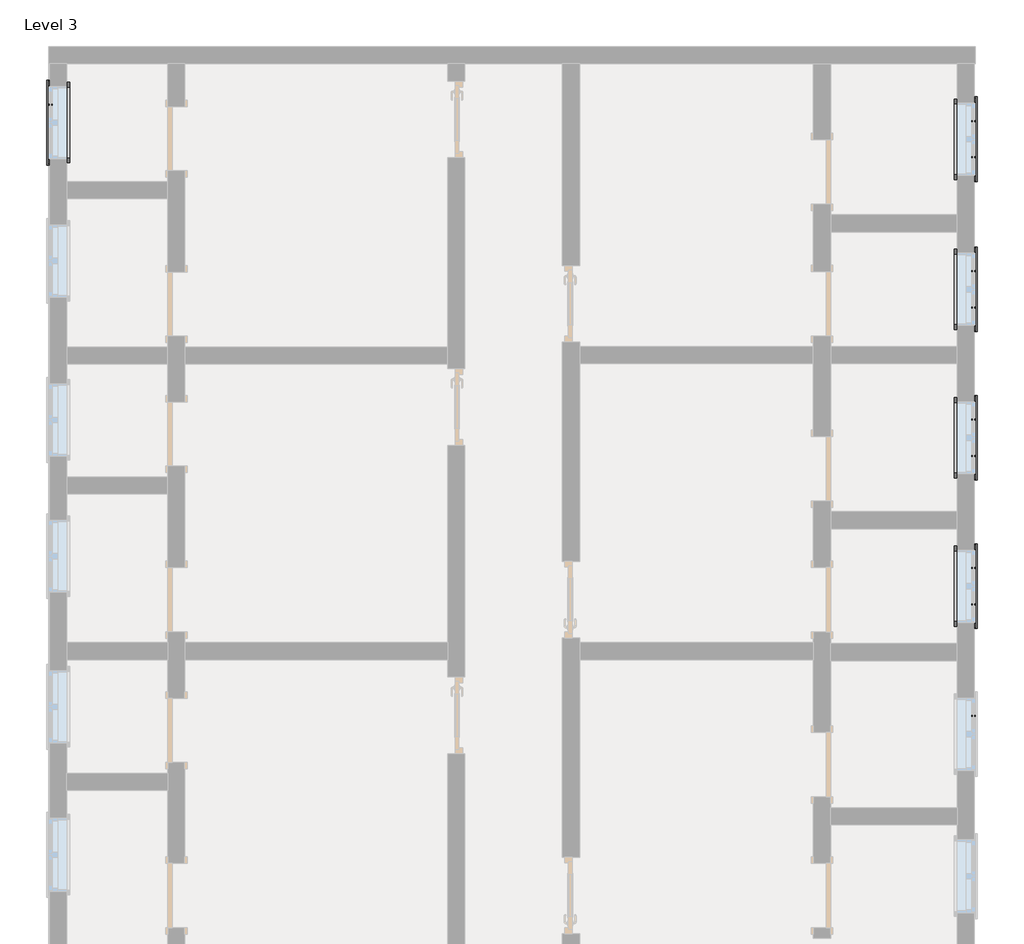
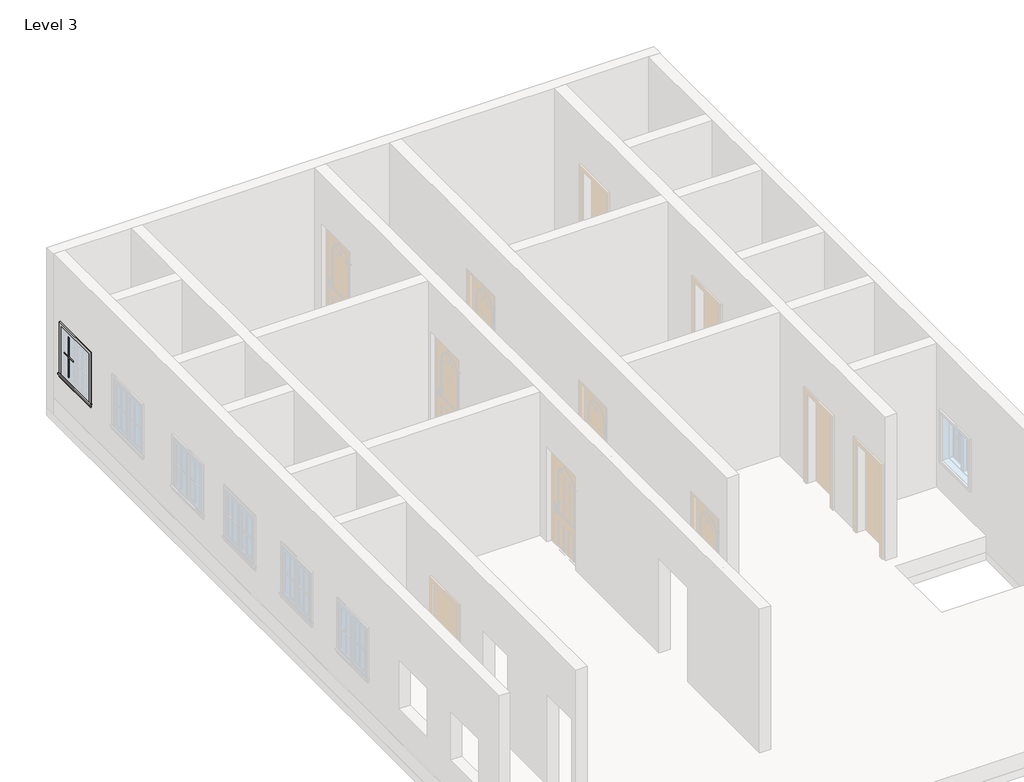
# One storey, part 4 of 4: 20 proxies.
"""IFC4 building model written with IfcOpenShell, lengths in millimetres."""

from ifc_helpers import new_model, si_unit, origin, place, context, project, spatial, transform, mapped, element, save
from components import muntin_pattern_2x2_muntin_pattern_2x2_b3fe6957, muntin_pattern_2x2_muntin_pattern_2x2_3e0ecaf2, trim_window_exterior_flat_with_sill_41619996, trim_window_interior_flat_picture_frame_51c85655

model = new_model("IFC4")

# Units and contexts
model_context = context("Model", 3, world=origin())
ifc_project = project(units=[si_unit("LENGTHUNIT", "METRE", prefix="MILLI")], contexts=[model_context])

# Site, building, storey
site = spatial("IfcSite", under=ifc_project)
building = spatial("IfcBuilding", under=site)
storey = spatial("IfcBuildingStorey", under=building, Name="Level 3", Elevation=6096.0)

# Proxies
placement = place(None, origin())
muntin_pattern_2x2_muntin_pattern_2x2_shape = muntin_pattern_2x2_muntin_pattern_2x2_b3fe6957(model_context)
element("IfcBuildingElementProxy", 1, Name="Muntin Pattern_2x2 : Muntin Pattern_2x2", ObjectType="Muntin Pattern_2x2 : Muntin Pattern_2x2", at=placement, inside=storey, context=model_context, shape_type="MappedRepresentation", body=[
    mapped(muntin_pattern_2x2_muntin_pattern_2x2_shape, transform((4489.4641134, 66.1024728, 7080.25), x_axis=(0.0, -1.0, 0.0), y_axis=(1.0, 0.0, 0.0), z_axis=(0.0, 0.0, 1.0))),
])
element("IfcBuildingElementProxy", 2, Name="Muntin Pattern_2x2 : Muntin Pattern_2x2", ObjectType="Muntin Pattern_2x2 : Muntin Pattern_2x2", at=placement, inside=storey, context=model_context, shape_type="MappedRepresentation", body=[
    mapped(muntin_pattern_2x2_muntin_pattern_2x2_shape, transform((4489.4641134, 1818.7024728, 7080.25), x_axis=(0.0, -1.0, 0.0), y_axis=(1.0, 0.0, 0.0), z_axis=(0.0, 0.0, 1.0))),
])
element("IfcBuildingElementProxy", 3, Name="Muntin Pattern_2x2 : Muntin Pattern_2x2", ObjectType="Muntin Pattern_2x2 : Muntin Pattern_2x2", at=placement, inside=storey, context=model_context, shape_type="MappedRepresentation", body=[
    mapped(muntin_pattern_2x2_muntin_pattern_2x2_shape, transform((4489.4641134, 3577.6524728, 7080.25), x_axis=(0.0, -1.0, 0.0), y_axis=(1.0, 0.0, 0.0), z_axis=(0.0, 0.0, 1.0))),
])
element("IfcBuildingElementProxy", 4, Name="Muntin Pattern_2x2 : Muntin Pattern_2x2", ObjectType="Muntin Pattern_2x2 : Muntin Pattern_2x2", at=placement, inside=storey, context=model_context, shape_type="MappedRepresentation", body=[
    mapped(muntin_pattern_2x2_muntin_pattern_2x2_shape, transform((4489.4641134, 5336.6024728, 7080.25), x_axis=(0.0, -1.0, 0.0), y_axis=(1.0, 0.0, 0.0), z_axis=(0.0, 0.0, 1.0))),
])
element("IfcBuildingElementProxy", 5, Name="Muntin Pattern_2x2 : Muntin Pattern_2x2", ObjectType="Muntin Pattern_2x2 : Muntin Pattern_2x2", at=placement, inside=storey, context=model_context, shape_type="MappedRepresentation", body=[
    mapped(muntin_pattern_2x2_muntin_pattern_2x2_shape, transform((4489.4641134, 7114.6024728, 7080.25), x_axis=(0.0, -1.0, 0.0), y_axis=(1.0, 0.0, 0.0), z_axis=(0.0, 0.0, 1.0))),
])
muntin_pattern_2x2_muntin_pattern_2x2_2_shape = muntin_pattern_2x2_muntin_pattern_2x2_3e0ecaf2(model_context)
element("IfcBuildingElementProxy", 6, Name="Muntin Pattern_2x2 : Muntin Pattern_2x2", ObjectType="Muntin Pattern_2x2 : Muntin Pattern_2x2", at=placement, inside=storey, context=model_context, shape_type="MappedRepresentation", body=[
    mapped(muntin_pattern_2x2_muntin_pattern_2x2_2_shape, transform((-6438.8858866, 7311.4524728, 7080.25), x_axis=(0.0, -1.0, 0.0), y_axis=(1.0, 0.0, 0.0), z_axis=(0.0, 0.0, 1.0))),
])
element("IfcBuildingElementProxy", 7, Name="Muntin Pattern_2x2 : Muntin Pattern_2x2", ObjectType="Muntin Pattern_2x2 : Muntin Pattern_2x2", at=placement, inside=storey, context=model_context, shape_type="MappedRepresentation", body=[
    mapped(muntin_pattern_2x2_muntin_pattern_2x2_2_shape, transform((4489.4641134, 1390.0774728, 7080.25), x_axis=(0.0, 1.0, 0.0), y_axis=(-1.0, 0.0, 0.0), z_axis=(0.0, 0.0, 1.0))),
])
element("IfcBuildingElementProxy", 8, Name="Muntin Pattern_2x2 : Muntin Pattern_2x2", ObjectType="Muntin Pattern_2x2 : Muntin Pattern_2x2", at=placement, inside=storey, context=model_context, shape_type="MappedRepresentation", body=[
    mapped(muntin_pattern_2x2_muntin_pattern_2x2_2_shape, transform((4489.4641134, 3149.0274728, 7080.25), x_axis=(0.0, 1.0, 0.0), y_axis=(-1.0, 0.0, 0.0), z_axis=(0.0, 0.0, 1.0))),
])
element("IfcBuildingElementProxy", 9, Name="Muntin Pattern_2x2 : Muntin Pattern_2x2", ObjectType="Muntin Pattern_2x2 : Muntin Pattern_2x2", at=placement, inside=storey, context=model_context, shape_type="MappedRepresentation", body=[
    mapped(muntin_pattern_2x2_muntin_pattern_2x2_2_shape, transform((4489.4641134, 4907.9774728, 7080.25), x_axis=(0.0, 1.0, 0.0), y_axis=(-1.0, 0.0, 0.0), z_axis=(0.0, 0.0, 1.0))),
])
element("IfcBuildingElementProxy", 10, Name="Muntin Pattern_2x2 : Muntin Pattern_2x2", ObjectType="Muntin Pattern_2x2 : Muntin Pattern_2x2", at=placement, inside=storey, context=model_context, shape_type="MappedRepresentation", body=[
    mapped(muntin_pattern_2x2_muntin_pattern_2x2_2_shape, transform((4489.4641134, 6685.9774728, 7080.25), x_axis=(0.0, 1.0, 0.0), y_axis=(-1.0, 0.0, 0.0), z_axis=(0.0, 0.0, 1.0))),
])
trim_window_exterior_flat_with_sill_shape = trim_window_exterior_flat_with_sill_41619996(model_context)
element("IfcBuildingElementProxy", 11, Name="Trim-Window-Exterior-Flat : with Sill", ObjectType="Trim-Window-Exterior-Flat : with Sill", at=placement, inside=storey, context=model_context, shape_type="MappedRepresentation", body=[
    mapped(trim_window_exterior_flat_with_sill_shape, transform((-6448.4108866, 7097.1399728, 7924.8), x_axis=(0.0, -1.0, 0.0), y_axis=(0.0, 0.0, 1.0), z_axis=(-1.0, 0.0, 0.0))),
])
element("IfcBuildingElementProxy", 12, Name="Trim-Window-Exterior-Flat : with Sill", ObjectType="Trim-Window-Exterior-Flat : with Sill", at=placement, inside=storey, context=model_context, shape_type="MappedRepresentation", body=[
    mapped(trim_window_exterior_flat_with_sill_shape, transform((4498.9891134, 1604.3899728, 7924.8), x_axis=(0.0, 1.0, 0.0), y_axis=(0.0, 0.0, 1.0), z_axis=(1.0, 0.0, 0.0))),
])
element("IfcBuildingElementProxy", 13, Name="Trim-Window-Exterior-Flat : with Sill", ObjectType="Trim-Window-Exterior-Flat : with Sill", at=placement, inside=storey, context=model_context, shape_type="MappedRepresentation", body=[
    mapped(trim_window_exterior_flat_with_sill_shape, transform((4498.9891134, 3363.3399728, 7924.8), x_axis=(0.0, 1.0, 0.0), y_axis=(0.0, 0.0, 1.0), z_axis=(1.0, 0.0, 0.0))),
])
element("IfcBuildingElementProxy", 14, Name="Trim-Window-Exterior-Flat : with Sill", ObjectType="Trim-Window-Exterior-Flat : with Sill", at=placement, inside=storey, context=model_context, shape_type="MappedRepresentation", body=[
    mapped(trim_window_exterior_flat_with_sill_shape, transform((4498.9891134, 5122.2899728, 7924.8), x_axis=(0.0, 1.0, 0.0), y_axis=(0.0, 0.0, 1.0), z_axis=(1.0, 0.0, 0.0))),
])
element("IfcBuildingElementProxy", 15, Name="Trim-Window-Exterior-Flat : with Sill", ObjectType="Trim-Window-Exterior-Flat : with Sill", at=placement, inside=storey, context=model_context, shape_type="MappedRepresentation", body=[
    mapped(trim_window_exterior_flat_with_sill_shape, transform((4498.9891134, 6900.2899728, 7924.8), x_axis=(0.0, 1.0, 0.0), y_axis=(0.0, 0.0, 1.0), z_axis=(1.0, 0.0, 0.0))),
])
trim_window_interior_flat_picture_frame_shape = trim_window_interior_flat_picture_frame_51c85655(model_context)
element("IfcBuildingElementProxy", 16, Name="Trim-Window-Interior-Flat : Picture Frame", ObjectType="Trim-Window-Interior-Flat : Picture Frame", at=placement, inside=storey, context=model_context, shape_type="MappedRepresentation", body=[
    mapped(trim_window_interior_flat_picture_frame_shape, transform((-6245.2108866, 7097.1399728, 7924.8), x_axis=(0.0, 1.0, 0.0), y_axis=(0.0, 0.0, 1.0), z_axis=(1.0, 0.0, 0.0))),
])
element("IfcBuildingElementProxy", 17, Name="Trim-Window-Interior-Flat : Picture Frame", ObjectType="Trim-Window-Interior-Flat : Picture Frame", at=placement, inside=storey, context=model_context, shape_type="MappedRepresentation", body=[
    mapped(trim_window_interior_flat_picture_frame_shape, transform((4295.7891134, 1604.3899728, 7924.8), x_axis=(0.0, -1.0, 0.0), y_axis=(0.0, 0.0, 1.0), z_axis=(-1.0, 0.0, 0.0))),
])
element("IfcBuildingElementProxy", 18, Name="Trim-Window-Interior-Flat : Picture Frame", ObjectType="Trim-Window-Interior-Flat : Picture Frame", at=placement, inside=storey, context=model_context, shape_type="MappedRepresentation", body=[
    mapped(trim_window_interior_flat_picture_frame_shape, transform((4295.7891134, 3363.3399728, 7924.8), x_axis=(0.0, -1.0, 0.0), y_axis=(0.0, 0.0, 1.0), z_axis=(-1.0, 0.0, 0.0))),
])
element("IfcBuildingElementProxy", 19, Name="Trim-Window-Interior-Flat : Picture Frame", ObjectType="Trim-Window-Interior-Flat : Picture Frame", at=placement, inside=storey, context=model_context, shape_type="MappedRepresentation", body=[
    mapped(trim_window_interior_flat_picture_frame_shape, transform((4295.7891134, 5122.2899728, 7924.8), x_axis=(0.0, -1.0, 0.0), y_axis=(0.0, 0.0, 1.0), z_axis=(-1.0, 0.0, 0.0))),
])
element("IfcBuildingElementProxy", 20, Name="Trim-Window-Interior-Flat : Picture Frame", ObjectType="Trim-Window-Interior-Flat : Picture Frame", at=placement, inside=storey, context=model_context, shape_type="MappedRepresentation", body=[
    mapped(trim_window_interior_flat_picture_frame_shape, transform((4295.7891134, 6900.2899728, 7924.8), x_axis=(0.0, -1.0, 0.0), y_axis=(0.0, 0.0, 1.0), z_axis=(-1.0, 0.0, 0.0))),
])

save(model, "model.ifc")

# Revit data of these elements
# Type "Muntin Pattern_2x2 : Muntin Pattern_2x2"
#   Width [instance default] = 4' - 0"
#   Thickness = 0' - 0 1/2"
#   Height [instance default] = 4' - 0"
#   Distance = 0' - 0 3/4"
#   Interior Material [instance default] = none
#   Exterior Material [instance default] = none
#   Default Elevation = 0
# Type "Trim-Window-Exterior-Flat : with Sill"
#   Trim Width = 0' - 2 1/4"
#   Trim Thickness_Picture Frame = 0' - 1 1/4"
#   Trim Thickness_with Sill = 0' - 0 3/4"
#   Sill Thickness = 0' - 1 1/4"
#   Opening Width [instance default] = 2' - 0"
#   Opening Height [instance default] = 3' - 0"
#   Default Elevation = 4' - 0"
#   Sill = yes
#   Picture Frame = no
#   Trim Material [instance default] = none
# Type "Trim-Window-Interior-Flat : Picture Frame"
#   Trim Thickness_Picture Frame = 0' - 1 1/4"
#   Trim Width = 0' - 2 1/4"
#   Trim Thickness_with Sill = 0' - 0 3/4"
#   Sill Thickness = 0' - 1 1/4"
#   Opening Width [instance default] = 2' - 0"
#   Opening Height [instance default] = 3' - 0"
#   Default Elevation = 4' - 0"
#   Sill = no
#   Picture Frame = yes
#   Trim Material [instance default] = none
# Elements 1, 2, 3, 4, 5, 6, 7, 8, 9, 10 (IfcBuildingElementProxy, "Muntin Pattern_2x2 : Muntin Pattern_2x2")
#   Width = 0' - 11 5/8"
#   Height = 2' - 6 1/2"
#   Interior Material = Wood - Stained
#   Exterior Material = Clad - White
#   Phase Created = New Construction
#   Materials on its faces: "Clad - White", "Wood - Stained"
# Elements 11, 12, 13, 14, 15 (IfcBuildingElementProxy, "Trim-Window-Exterior-Flat : with Sill")
#   Opening Width = 2' - 10"
#   Opening Height = 3' - 0"
#   Trim Material = Clad - White
#   Phase Created = New Construction
#   Materials on its faces: "Clad - White"
# Elements 16, 17, 18, 19, 20 (IfcBuildingElementProxy, "Trim-Window-Interior-Flat : Picture Frame")
#   Opening Width = 2' - 10"
#   Opening Height = 3' - 0"
#   Trim Material = Wood - Stained
#   Phase Created = New Construction
#   Materials on its faces: "Wood - Stained"
# Materials
#   "Clad - White": class "Wood", colour RGB 242 242 238, transparency 0, Cost = 0
#   "Wood - Stained": class "Wood", colour RGB 224 178 126, transparency 0, Cost = 0
